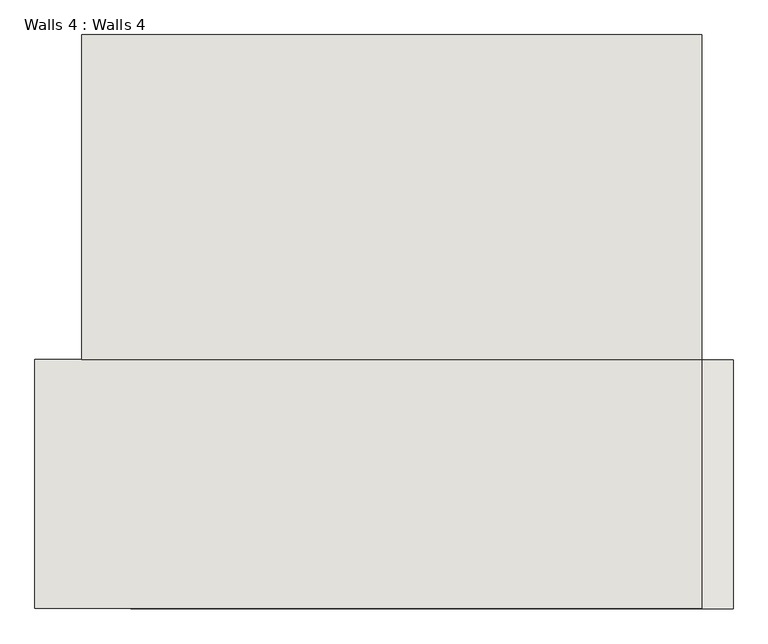
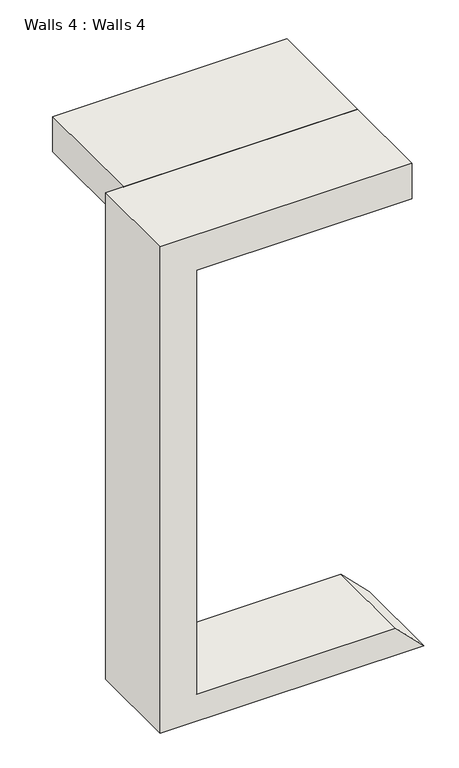
"""IFC4 building model written with IfcOpenShell, lengths in millimetres: wall geometry, Walls 4 : Walls 4."""

from ifc_helpers import new_model, si_unit, frame, origin, place, context, project, spatial, polyline, outline, extrude, source, transform, mapped, element, save


def walls_4_walls_4_fad0a3e8(model_context):
    return source(origin(), model_context, "Body", "SweptSolid", [
        extrude(outline(polyline([(-2140.3749149, -2002.282557), (-5010.5749149, -2002.282557), (-5010.5749149, -497.7209011), (-2140.3749149, -497.7209011), (-2140.3749149, -2002.282557)])), frame((0.0, 0.0, 17830.8), z_axis=(0.0, 0.0, 1.0), x_axis=(1.0, 0.0, 0.0)), (0.0, 0.0, 1.0), 457.2),
        extrude(outline(polyline([(11995.15, -5226.4749149), (11995.15, -1994.3249149), (12344.4, -2343.5749149), (12344.4, -4781.9749149), (17830.8, -4781.9749149), (17830.8, -2140.3749149), (18288.0, -2140.3749149), (18288.0, -5226.4749149), (11995.15, -5226.4749149)])), frame((0.0, -3155.3872058, 0.0), z_axis=(0.0, 1.0, 0.0), x_axis=(0.0, 0.0, 1.0)), (0.0, 0.0, 1.0), 1153.1046488),
    ])


if __name__ == "__main__":
    model = new_model("IFC4")
    model_context = context("Model", 3, world=origin())
    ifc_project = project(units=[si_unit("LENGTHUNIT", "METRE", prefix="MILLI")], contexts=[model_context])
    site = spatial("IfcSite", under=ifc_project)
    building = spatial("IfcBuilding", under=site)
    placement = place(None, origin())
    walls_4_walls_4_shape = walls_4_walls_4_fad0a3e8(model_context)
    element("IfcWall", 1, ObjectType="Walls 4 : Walls 4", at=placement, inside=building, context=model_context, shape_type="MappedRepresentation", body=[
        mapped(walls_4_walls_4_shape, transform((0.0, 0.0, 0.0), x_axis=(1.0, 0.0, 0.0), y_axis=(0.0, 1.0, 0.0), z_axis=(0.0, 0.0, 1.0))),
    ])
    save(model, "model.ifc")

# Revit data of these elements
# Element 1 (IfcWall, "Walls 4 : Walls 4")
#   Materials on its faces: "Default Wall"
# Materials
#   "Default Wall": colour RGB 128 128 128, transparency 0
